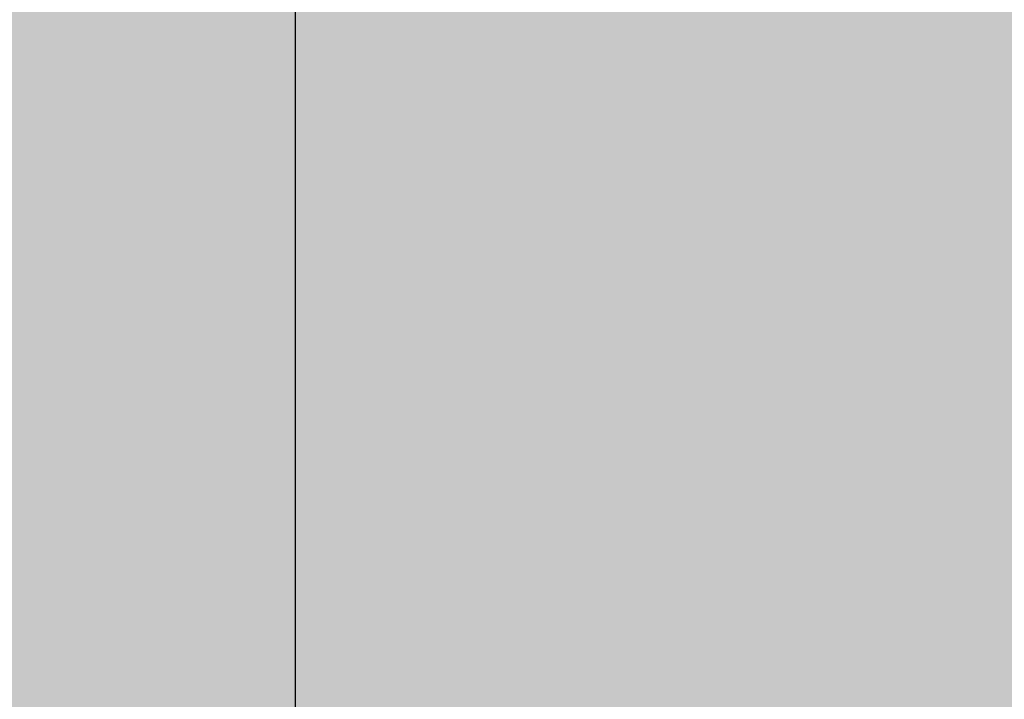
# Model space of a CAD drawing. Units: inches. Extents: x 2083 to 3317, y 1141 to 2115.
# Tile 26 of 256: x 2235.9182 to 2236.0667, y 1477.6562 to 1477.7587. Entities that reach past the tile are written whole.
import ezdxf

# ---------------------------------------------------------------- set-up
doc = ezdxf.new("R2010")
doc.units = ezdxf.units.IN
doc.layers.add('A-ANNO-DIMS', color=2, linetype='Continuous', lineweight=18)
doc.layers.add('A-WALL-PATT', color=251, linetype='Continuous', lineweight=13, true_color=0x636466)
doc.styles.get("Standard").update_dxf_attribs({"font": 'arial.ttf'})
doc.dimstyles.new('ISO-25', dxfattribs={"dimtxt": 12, "dimasz": 12, "dimexe": 1.25, "dimexo": 0.625, "dimtad": 1, "dimlunit": 3, "dimtxsty": 'Standard', "dimcen": 2.5, "dimadec": 0, "dimazin": 0, "dimtfac": 1, "dimtmove": 0, "dimatfit": 3, "dimfxl": 1, "dimarcsym": 0})

# ---------------------------------------------------------------- blocks, each defined once
blk = doc.blocks.new('*D30')
at = {"layer": 'A-ANNO-DIMS', "color": 0, "lineweight": -2, "transparency": 16777216}
for p, q in [((2240.01786, 1445.27381), (2240.01786, 1448.04553)), ((2254.32933, 1445.27381), (2254.32933, 1448.04553)), ((2228.01786, 1446.79553), (2216.01786, 1446.79553)), ((2240.01786, 1446.79553), (2254.32933, 1446.79553)), ((2266.32933, 1446.79553), (2413.76487, 1446.79553))]:
    blk.add_line(p, q, dxfattribs=at)
at = {"layer": 'A-ANNO-DIMS', "color": 0, "transparency": 16777216}
for points in [[(2228.01786, 1448.79553), (2228.01786, 1444.79553), (2240.01786, 1446.79553)], [(2266.32933, 1448.79553), (2266.32933, 1444.79553), (2254.32933, 1446.79553)]]:
    blk.add_solid(points, dxfattribs=at)
at = {"layer": 'Defpoints', "color": 0, "transparency": 16777216}
for p in [(2254.32933, 1446.79553), (2240.01786, 1444.64881), (2254.32933, 1444.64881)]:
    blk.add_point(p, dxfattribs=at)
at = {"layer": 'A-ANNO-DIMS', "color": 0, "transparency": 16777216, "insert": (2346.0471, 1453.62517), "char_height": 12, "attachment_point": 5}
blk.add_mtext('WC 1\'-2 1/2" TYP.', dxfattribs=at)
blk = doc.blocks.new('*D31')
at = {"layer": 'A-ANNO-DIMS', "color": 0, "lineweight": -2, "transparency": 16777216}
for p, q in [((2237.87114, 1456.64881), (2237.87114, 1541.91518)), ((2239.39286, 1444.64881), (2236.62114, 1444.64881)), ((2237.87114, 1431.54754), (2237.87114, 1444.64881)), ((2239.39286, 1431.54754), (2236.62114, 1431.54754)), ((2237.87114, 1419.54754), (2237.87114, 1407.54754))]:
    blk.add_line(p, q, dxfattribs=at)
at = {"layer": 'A-ANNO-DIMS', "color": 0, "transparency": 16777216}
for points in [[(2235.87114, 1456.64881), (2239.87114, 1456.64881), (2237.87114, 1444.64881)], [(2235.87114, 1419.54754), (2239.87114, 1419.54754), (2237.87114, 1431.54754)]]:
    blk.add_solid(points, dxfattribs=at)
at = {"layer": 'Defpoints', "color": 0, "transparency": 16777216}
for p in [(2237.87114, 1444.64881), (2240.01786, 1444.64881), (2240.01786, 1431.54754)]:
    blk.add_point(p, dxfattribs=at)
at = {"layer": 'A-ANNO-DIMS', "color": 0, "transparency": 16777216, "insert": (2231.21749, 1505.28199), "char_height": 12, "attachment_point": 5, "rotation": 90}
blk.add_mtext('1\'-1" TYP.', dxfattribs=at)
blk = doc.blocks.new('*D62')
at = {"layer": 'A-ANNO-DIMS', "color": 0, "lineweight": -2, "transparency": 16777216}
for p, q in [((2235.95978, 1469.38636), (2235.95978, 1522.36136)), ((2379.95978, 1469.38636), (2379.95978, 1522.36136)), ((2247.95978, 1521.11136), (2367.95978, 1521.11136))]:
    blk.add_line(p, q, dxfattribs=at)
at = {"layer": 'A-ANNO-DIMS', "color": 0, "transparency": 16777216}
for points in [[(2247.95978, 1523.11136), (2247.95978, 1519.11136), (2235.95978, 1521.11136)], [(2367.95978, 1523.11136), (2367.95978, 1519.11136), (2379.95978, 1521.11136)]]:
    blk.add_solid(points, dxfattribs=at)
at = {"layer": 'Defpoints', "color": 0, "transparency": 16777216}
for p in [(2379.95978, 1521.11136), (2235.95978, 1468.76136), (2379.95978, 1468.76136)]:
    blk.add_point(p, dxfattribs=at)
at = {"layer": 'A-ANNO-DIMS', "color": 0, "transparency": 16777216, "insert": (2307.95978, 1527.86324), "char_height": 12, "attachment_point": 5}
blk.add_mtext('12\'-0"', dxfattribs=at)

msp = doc.modelspace()

# ---------------------------------------------------------------- hatches: boundary and pattern name
at = {"layer": 'A-WALL-PATT'}
h = msp.add_hatch(color=256, dxfattribs=at)
h.dxf.hatch_style = 1
h.paths.add_polyline_path([(3126.95978, 2020.76136), (2748.95978, 2020.76136), (2604.95978, 2020.76136), (2226.95978, 2020.76136), (2226.95978, 1702.76136), (2466.95978, 1702.76136), (2466.95978, 1582.76136), (2418.95978, 1582.76136), (2418.95978, 1477.76136), (2226.95978, 1477.76136), (2226.95978, 1263.26136), (2544.95978, 1263.26136), (2544.95978, 1411.76136), (2604.95978, 1411.76136), (2685.95978, 1411.76136), (2685.95978, 1420.76136), (2604.95978, 1420.76136), (2604.95978, 1573.76136), (2604.95978, 1702.76136), (2604.95978, 2011.76136), (2748.95978, 2011.76136), (2748.95978, 1702.76136), (2862.95978, 1702.76136), (2862.95978, 1621.76136), (2871.95978, 1621.76136), (2871.95978, 1702.76136), (2883.95978, 1702.76136), (2883.95978, 1706.93946, -0.026459), (2883.95978, 1711.76136), (2757.95978, 1711.76136), (2757.95978, 1807.76136), (2787.95978, 1807.76136), (2787.95978, 1812.26136), (2757.95978, 1812.26136), (2757.95978, 2011.76136), (2877.95978, 2011.76136), (2877.95978, 1812.26136), (2847.95978, 1812.26136), (2847.95978, 1807.76136), (2889.83574, 1807.76136), (2889.83574, 1812.26136), (2882.45978, 1812.26136), (2882.45978, 2011.76136), (3117.95978, 2011.76136), (3117.95978, 1812.26136), (2937.83574, 1812.26136), (2937.83574, 1807.76136), (2995.70978, 1807.76136), (2995.70978, 1796.11767), (3000.20978, 1796.11767), (3000.20978, 1807.76136), (3117.95978, 1807.76136), (3117.95978, 1711.76136), (3000.20978, 1711.76136), (3000.20978, 1760.11767), (2998.5727, 1760.11767, -0.020711), (2995.70978, 1760.11767), (2995.70978, 1711.76136), (2931.95978, 1711.76136), (2931.95978, 1702.76136), (3126.95978, 1702.76136)])
h.paths.add_polyline_path([(2471.45978, 2011.76136), (2471.45978, 1810.01136), (2462.71694, 1810.01136), (2462.71694, 1805.51136), (2505.95978, 1805.51136), (2505.95978, 1810.01136), (2475.95978, 1810.01136), (2475.95978, 2011.76136), (2595.95978, 2011.76136), (2595.95978, 1810.01136), (2565.95978, 1810.01136), (2565.95978, 1805.51136), (2595.95978, 1805.51136), (2595.95978, 1711.76136), (2235.95978, 1711.76136), (2235.95978, 1805.51136), (2353.70978, 1805.51136), (2353.70978, 1796.05416), (2358.20978, 1796.05416), (2358.20978, 1805.51136), (2414.71694, 1805.51136), (2414.71694, 1810.01136), (2235.95978, 1810.01136), (2235.95978, 2011.76136)], flags=16)
h.paths.add_polyline_path([(2270.20473, 1994.61001), (2270.20473, 1970.61001), (2246.20473, 1970.61001), (2246.20473, 1994.61001)], flags=0)
edge = h.paths.add_edge_path(flags=0)
edge.add_ellipse((2332.02739, 1899.79818), major_axis=(-3.04299, 3.04299), ratio=0.1682525, start_angle=-161.33217, end_angle=-156.30711, ccw=False)
edge.add_ellipse((2333.08204, 1898.74353), major_axis=(-1.05465, 1.05465), ratio=0.4535321, start_angle=-123.37102, end_angle=-94.15911)
edge = h.paths.add_edge_path(flags=0)
edge.add_ellipse((2332.02739, 1968.87629), major_axis=(3.04299, 3.04299), ratio=0.1682525, start_angle=18.66783, end_angle=23.69289)
edge.add_spline(control_points=[(2332.9256, 1970.6911), (2332.22677, 1970.3361), (2330.89371, 1969.65891), (2328.41308, 1970.93214), (2327.20393, 1967.74871), (2324.7096, 1969.95559), (2322.53282, 1967.01235), (2320.01285, 1971.29581), (2317.68031, 1968.15784), (2316.04053, 1967.10205), (2315.4269, 1966.8096)], knot_values=[0, 0, 0, 0, 2.267059, 4.324559, 6.685584, 8.878641, 11.121502, 14.300359, 17.755284, 19.732645, 19.732645, 19.732645, 19.732645], degree=3, periodic=0)
edge.add_ellipse((2332.02739, 1968.87629), major_axis=(3.04299, 3.04299), ratio=0.1682525, start_angle=18.66783, end_angle=23.69289, ccw=False)
edge.add_ellipse((2333.08204, 1969.93094), major_axis=(1.05465, 1.05465), ratio=0.4535321, start_angle=56.62898, end_angle=85.84089, ccw=False)
edge = h.paths.add_edge_path(flags=0)
edge.add_spline(control_points=[(2296.42829, 1967.98791), (2293.6278, 1965.33631), (2287.70362, 1959.72709), (2299.74386, 1949.9957), (2294.53259, 1935.66853), (2290.57323, 1920.60351), (2293.39412, 1909.97369), (2296.18541, 1904.96654)], knot_values=[0.099185, 0.099185, 0.099185, 0.099185, 0.345301, 0.619822, 0.982653, 1.386093, 1.810555, 1.810555, 1.810555, 1.810555], degree=3, periodic=0)
edge.add_spline(control_points=[(2296.18541, 1904.96654), (2297.38358, 1902.6193), (2298.00097, 1901.94931), (2298.55297, 1901.46815)], knot_values=[0.006246, 0.006246, 0.006246, 0.006246, 0.055476, 0.055476, 0.055476, 0.055476], degree=3, periodic=0)
edge.add_spline(control_points=[(2298.55297, 1901.46815), (2297.25861, 1900.92322), (2295.22529, 1900.23213), (2293.06023, 1900.61421), (2292.10142, 1900.78841), (2292.08958, 1900.79057)], knot_values=[0.312835, 0.312835, 0.312835, 0.312835, 0.40178, 0.474987, 0.475903, 0.475903, 0.475903, 0.475903], degree=3, periodic=0)
edge.add_arc((2292.79365, 1904.66411), 3.93701, 215.4209, 259.69818, ccw=False)
edge.add_spline(control_points=[(2289.58531, 1902.3823), (2289.47665, 1902.53509), (2289.36848, 1902.68804), (2289.26086, 1902.84117)], knot_values=[0.102872, 0.102872, 0.102872, 0.102872, 0.116896, 0.116896, 0.116896, 0.116896], degree=3, periodic=0)
edge.add_spline(control_points=[(2289.26086, 1902.84117), (2288.6866, 1902.55019), (2287.64005, 1902.0199), (2285.88134, 1901.87395), (2283.85297, 1901.50435), (2281.71999, 1899.71054), (2278.46699, 1899.49294), (2276.15714, 1901.8832), (2272.25895, 1899.80407), (2267.77761, 1901.84318), (2262.24388, 1900.18403), (2257.41493, 1901.78206), (2254.31837, 1900.72612), (2253.17828, 1900.33734)], knot_values=[0, 0, 0, 0, 1.907977, 3.477176, 5.261074, 7.972851, 11.680248, 13.717921, 16.939592, 22.789562, 27.502503, 33.595215, 37.145618, 37.145618, 37.145618, 37.145618], degree=3, periodic=0)
edge.add_line((2253.17828, 1900.33734), (2250.24424, 1902.84117))
edge.add_line((2250.24424, 1902.84117), (2250.24424, 1965.8333))
edge.add_line((2250.24424, 1965.8333), (2253.17828, 1968.33712))
edge.add_spline(control_points=[(2253.17828, 1968.33712), (2254.31837, 1967.94835), (2257.41493, 1966.89241), (2262.24388, 1968.49043), (2267.77761, 1966.83128), (2271.52673, 1968.53722), (2273.87591, 1967.82829), (2274.2067, 1967.72764)], knot_values=[0, 0, 0, 0, 0.09018, 0.244935, 0.364644, 0.513233, 0.537855, 0.537855, 0.537855, 0.537855], degree=3, periodic=0)
edge.add_arc((2274.35289, 1963.79335), 3.93701, 72.05113, 92.12795, ccw=False)
edge.add_arc((2281.29693, 1985.23), 18.5963, 252.051134, 288.565722)
edge.add_arc((2292.31672, 1956.02888), 12.64608, 71.026788, 113.778218, ccw=False)
edge = h.paths.add_edge_path(flags=0)
edge.add_spline(control_points=[(2274.89941, 1951.85619), (2275.06616, 1951.61659), (2275.23269, 1951.37659), (2275.39799, 1951.13585)], knot_values=[1.409916, 1.409916, 1.409916, 1.409916, 1.43159, 1.43159, 1.43159, 1.43159], degree=3, periodic=0)
edge.add_spline(control_points=[(2275.39799, 1951.13585), (2275.79211, 1950.56189), (2276.17923, 1949.98377), (2276.54555, 1949.3971)], knot_values=[1.358238, 1.358238, 1.358238, 1.358238, 1.409916, 1.409916, 1.409916, 1.409916], degree=3, periodic=0)
edge.add_line((2276.54555, 1949.3971), (2277.43729, 1947.86218))
edge.add_spline(control_points=[(2277.43729, 1947.86218), (2276.30383, 1945.67311), (2274.6397, 1942.42688), (2274.63161, 1938.0939), (2272.79912, 1930.85155), (2274.35643, 1943.89705), (2275.94768, 1947.92336), (2276.54555, 1949.3971)], knot_values=[0.005632, 0.005632, 0.005632, 0.005632, 0.186014, 0.266002, 0.357087, 0.59639, 0.739732, 0.739732, 0.739732, 0.739732], degree=3, periodic=0)
edge.add_spline(control_points=[(2276.54555, 1949.3971), (2276.17923, 1949.98377), (2275.79211, 1950.56189), (2275.39799, 1951.13585)], knot_values=[1.358238, 1.358238, 1.358238, 1.358238, 1.409916, 1.409916, 1.409916, 1.409916], degree=3, periodic=0)
edge.add_spline(control_points=[(2275.39799, 1951.13585), (2274.9425, 1950.08045), (2274.20776, 1948.02527), (2273.9346, 1944.85148), (2272.46853, 1937.62749), (2273.46622, 1945.69647), (2274.70062, 1951.05947), (2274.89941, 1951.85619)], knot_values=[0.104364, 0.104364, 0.104364, 0.104364, 0.189636, 0.269624, 0.36071, 0.600013, 0.644622, 0.644622, 0.644622, 0.644622], degree=3, periodic=0)
h.paths.add_polyline_path([(2269.16751, 1963.12757, -0.357527), (2268.17063, 1960.97637, -0.092561), (2268.17063, 1939.43632, -0.357527), (2269.16751, 1937.28512, -0.357527), (2267.01631, 1938.282, -0.164785), (2254.68558, 1938.282, -0.357527), (2252.53438, 1937.28512, -0.357527), (2253.53126, 1939.43632, -0.092561), (2253.53126, 1960.97637, -0.357527), (2252.53438, 1963.12757, -0.357527), (2254.68558, 1962.13069, -0.164785), (2267.01631, 1962.13069, -0.357527)], flags=0)
h.paths.add_polyline_path([(2248.87407, 1967.8018), (2248.87407, 1957.02771), (2249.45778, 1957.02771), (2249.45778, 1911.64676), (2248.87407, 1911.64676), (2248.87407, 1900.87267), (2246.51186, 1900.87267, 0.197327), (2244.14966, 1902.45687), (2244.14966, 1966.21759, 0.197327), (2246.51186, 1967.8018)], flags=0)
h.paths.add_polyline_path([(2269.16751, 1931.38934, -0.357527), (2268.17063, 1929.23814, -0.092561), (2268.17063, 1907.6981, -0.357527), (2269.16751, 1905.54689, -0.357527), (2267.01631, 1906.54377, -0.164785), (2254.68558, 1906.54377, -0.357527), (2252.53438, 1905.54689, -0.357527), (2253.53126, 1907.6981, -0.092561), (2253.53126, 1929.23814, -0.357527), (2252.53438, 1931.38934, -0.357527), (2254.68558, 1930.39246, -0.164785), (2267.01631, 1930.39246, -0.357527)], flags=0)
edge = h.paths.add_edge_path(flags=0)
edge.add_spline(control_points=[(2276.19686, 1906.7237), (2276.16814, 1909.02893), (2276.11405, 1913.37185), (2270.59842, 1924.92498), (2273.90517, 1919.01278), (2275.92171, 1916.26206), (2275.47457, 1912.40215), (2277.25787, 1910.38062), (2276.69604, 1908.22504), (2276.64622, 1906.81302), (2276.61782, 1906.00841)], knot_values=[0, 0, 0, 0, 8.61026, 16.221274, 18.843057, 23.804898, 27.440828, 29.356102, 31.203478, 33.650687, 33.650687, 33.650687, 33.650687], degree=3, periodic=0)
edge.add_spline(control_points=[(2276.61782, 1906.00841), (2276.62331, 1905.62414), (2276.49774, 1904.62866), (2275.44178, 1903.85473), (2274.93731, 1903.08045), (2274.85908, 1902.84117)], knot_values=[0.156488, 0.156488, 0.156488, 0.156488, 0.184398, 0.231376, 0.250598, 0.250598, 0.250598, 0.250598], degree=3, periodic=0)
edge.add_line((2274.85908, 1902.84117), (2276.50598, 1902.84117))
edge.add_spline(control_points=[(2276.50598, 1902.84117), (2276.78831, 1903.08494), (2277.66507, 1904.1252), (2278.24954, 1904.34074), (2277.65387, 1908.52739), (2278.15567, 1906.22781), (2278.10046, 1905.28595), (2278.84667, 1904.06901), (2277.85679, 1903.41495), (2277.87419, 1902.99105), (2277.90356, 1902.84117)], knot_values=[0.059574, 0.059574, 0.059574, 0.059574, 0.080753, 0.103741, 0.16972, 0.176036, 0.207137, 0.240474, 0.262341, 0.27366, 0.27366, 0.27366, 0.27366], degree=3, periodic=0)
edge.add_line((2277.90356, 1902.84117), (2280.02983, 1902.84117))
edge.add_spline(control_points=[(2280.02983, 1902.84117), (2279.88822, 1903.0884), (2279.49926, 1903.98155), (2280.15228, 1905.93935), (2278.10362, 1909.65776), (2279.76239, 1907.18529), (2280.3279, 1904.87486), (2280.48511, 1903.48959), (2281.46327, 1903.24943), (2281.75834, 1902.9365), (2281.83404, 1902.84117)], knot_values=[0.013856, 0.013856, 0.013856, 0.013856, 0.034874, 0.088867, 0.107879, 0.126738, 0.158714, 0.193757, 0.217487, 0.226722, 0.226722, 0.226722, 0.226722], degree=3, periodic=0)
edge.add_spline(control_points=[(2281.83404, 1902.84117), (2281.78753, 1902.8267), (2281.64702, 1902.78299), (2281.39553, 1902.85949), (2281.08808, 1902.98524), (2280.72068, 1903.0609), (2280.33345, 1903.02573), (2280.12477, 1902.89888), (2280.02983, 1902.84117)], knot_values=[0, 0, 0, 0, 0.14413, 0.435517, 0.749276, 1.153046, 1.548371, 1.878348, 1.878348, 1.878348, 1.878348], degree=3, periodic=0)
edge.add_line((2280.02983, 1902.84117), (2277.90356, 1902.84117))
edge.add_spline(control_points=[(2277.90356, 1902.84117), (2277.89286, 1902.79586), (2277.8654, 1902.67964), (2277.60748, 1902.68748), (2277.27405, 1902.8007), (2276.83792, 1902.61977), (2276.58381, 1902.78926), (2276.50598, 1902.84117)], knot_values=[0, 0, 0, 0, 0.127189, 0.326199, 0.628009, 1.24357, 1.515331, 1.515331, 1.515331, 1.515331], degree=3, periodic=0)
edge.add_line((2276.50598, 1902.84117), (2274.85908, 1902.84117))
edge.add_spline(control_points=[(2274.85908, 1902.84117), (2274.81444, 1902.89859), (2274.72513, 1903.01345), (2274.49348, 1903.11897), (2274.24429, 1902.96054), (2273.93712, 1903.18494), (2273.61404, 1902.98314), (2273.40832, 1902.88304), (2273.32225, 1902.84117)], knot_values=[0, 0, 0, 0, 0.21843, 0.436957, 0.687977, 0.990379, 1.398396, 1.69185, 1.69185, 1.69185, 1.69185], degree=3, periodic=0)
edge.add_spline(control_points=[(2273.32225, 1902.84117), (2273.61674, 1903.44569), (2274.274, 1904.53825), (2276.02724, 1904.5737), (2276.20696, 1906.58364), (2276.19686, 1906.7237)], knot_values=[0.012227, 0.012227, 0.012227, 0.012227, 0.059472, 0.106218, 0.134458, 0.134458, 0.134458, 0.134458], degree=3, periodic=0)
h.paths.add_polyline_path([(2270.77605, 1897.78983), (2270.77605, 1873.78983), (2246.77605, 1873.78983), (2246.77605, 1897.78983)], flags=0)
h.paths.add_polyline_path([(2353.70978, 1760.00506), (2353.70978, 1760.05416), (2358.20978, 1760.05416, -0.033729)], flags=0)
h.paths.add_polyline_path([(2321.81912, 1737.52919), (2341.99533, 1737.52919, -0.414214), (2343.20327, 1736.32124), (2343.20327, 1721.0206, -0.414214), (2341.99533, 1719.81265), (2321.81912, 1719.81265, -0.414214), (2320.61117, 1721.0206), (2320.61117, 1736.32124, -0.414214)], flags=0)
h.paths.add_polyline_path([(2324.23501, 1736.32124), (2339.57944, 1736.32124, -0.414214), (2341.99533, 1733.90535), (2341.99533, 1725.44973, -0.414214), (2339.57944, 1723.03384), (2333.68059, 1723.03384), (2333.84532, 1722.04547, -0.870646), (2335.4254, 1721.82589, -0.767327), (2333.92269, 1721.42324), (2331.29102, 1721.42324, -0.767327), (2329.78832, 1721.82589, -0.870646), (2331.3684, 1722.04547), (2331.53313, 1723.03384), (2324.23501, 1723.03384, -0.414214), (2321.81912, 1725.44973), (2321.81912, 1733.90535, -0.414214)], flags=0)
h.paths.add_polyline_path([(2570.48379, 1928.61544), (2589.68379, 1928.61544), (2590.16883, 1928.61544), (2590.16883, 1904.9934), (2570.48379, 1904.9934)], flags=0)
h.paths.add_polyline_path([(2574.44732, 1927.26382, -1), (2572.82884, 1927.26382, -1)], flags=0)
h.paths.add_polyline_path([(2573.08987, 1926.94088), (2573.92503, 1927.77604), (2574.14774, 1927.55333), (2573.31258, 1926.71817)], flags=0)
h.paths.add_polyline_path([(2578.77906, 1919.72962, -1), (2571.59166, 1919.72962, -1)], flags=0)
h.paths.add_polyline_path([(2578.38536, 1919.72962, -1), (2571.98536, 1919.72962, -1)], flags=0)
h.paths.add_polyline_path([(2331.59576, 1729.47622, -1), (2333.61795, 1729.47622, -1)], flags=0)
h.paths.add_polyline_path([(2578.03423, 1927.26382, -1), (2576.41574, 1927.26382, -1)], flags=0)
h.paths.add_polyline_path([(2576.68885, 1927.53109), (2576.91156, 1927.7538), (2577.74673, 1926.91863), (2577.52402, 1926.69592)], flags=0)
h.paths.add_polyline_path([(2578.13906, 1909.85954, -1), (2572.23166, 1909.85954, -1)], flags=0)
h.paths.add_polyline_path([(2577.74536, 1909.85954, -1), (2572.62536, 1909.85954, -1)], flags=0)
h.paths.add_polyline_path([(2583.79772, 1927.26382, -1), (2582.17923, 1927.26382, -1)], flags=0)
h.paths.add_polyline_path([(2582.71865, 1927.7538), (2583.55381, 1926.91863), (2583.3311, 1926.69592), (2582.49594, 1927.53109)], flags=0)
h.paths.add_polyline_path([(2582.49594, 1927.53109), (2582.71865, 1927.7538), (2583.55381, 1926.91863), (2583.3311, 1926.69592)], flags=0)
h.paths.add_polyline_path([(2587.73906, 1920.52962, -1), (2581.83166, 1920.52962, -1)], flags=0)
h.paths.add_polyline_path([(2587.34536, 1920.52962, -1), (2582.22536, 1920.52962, -1)], flags=0)
h.paths.add_polyline_path([(2587.38462, 1927.26382, -1), (2585.76613, 1927.26382, -1)], flags=0)
h.paths.add_polyline_path([(2586.08199, 1926.98025), (2586.91716, 1927.81541), (2587.13987, 1927.5927), (2586.3047, 1926.75754)], flags=0)
h.paths.add_polyline_path([(2588.37906, 1910.65954, -1), (2581.19166, 1910.65954, -1)], flags=0)
h.paths.add_polyline_path([(2587.98536, 1910.65954, -1), (2581.58536, 1910.65954, -1)], flags=0)
h.paths.add_polyline_path([(2417.16773, 1729.4779), (2437.34394, 1729.4779, -0.414214), (2438.55188, 1728.26995), (2438.55188, 1712.96931, -0.414214), (2437.34394, 1711.76136), (2417.16773, 1711.76136, -0.414214), (2415.95978, 1712.96931), (2415.95978, 1728.26995, -0.414214)], flags=0)
h.paths.add_polyline_path([(2419.58362, 1728.26995), (2434.92805, 1728.26995, -0.414214), (2437.34394, 1725.85406), (2437.34394, 1717.39844, -0.414214), (2434.92805, 1714.98255), (2429.0292, 1714.98255), (2429.19393, 1713.99418, -0.870646), (2430.77401, 1713.7746, -0.767327), (2429.2713, 1713.37195), (2426.63963, 1713.37195, -0.767327), (2425.13693, 1713.7746, -0.870646), (2426.71701, 1713.99418), (2426.88174, 1714.98255), (2419.58362, 1714.98255, -0.414214), (2417.16773, 1717.39844), (2417.16773, 1725.85406, -0.414214)], flags=0)
h.paths.add_polyline_path([(2419.58362, 1728.26995), (2434.92805, 1728.26995, -0.414214), (2437.34394, 1725.85406), (2437.34394, 1717.39844, -0.414214), (2434.92805, 1714.98255), (2429.0292, 1714.98255), (2428.35812, 1719.00903), (2427.55282, 1719.00903), (2426.88174, 1714.98255), (2419.58362, 1714.98255, -0.414214), (2417.16773, 1717.39844), (2417.16773, 1725.85406, -0.414214)], flags=0)
h.paths.add_polyline_path([(2426.94437, 1721.42492, -1), (2428.96656, 1721.42492, -1)], flags=0)
h.paths.add_polyline_path([(2475.95978, 1702.76136), (2595.95978, 1702.76136), (2595.95978, 1582.76136), (2475.95978, 1582.76136)], flags=16)
h.paths.add_polyline_path([(2427.95978, 1573.76136), (2595.95978, 1573.76136), (2595.95978, 1468.76136), (2595.95978, 1420.76136), (2384.45978, 1420.76136), (2384.45978, 1468.76136), (2427.95978, 1468.76136)], flags=16)
h.paths.add_polyline_path([(2379.95978, 1468.76136), (2379.95978, 1420.76136), (2235.95978, 1420.76136), (2235.95978, 1468.76136)], flags=16)
h.paths.add_polyline_path([(2317.816, 1466.69577), (2337.9922, 1466.69577, -0.414214), (2339.20015, 1465.48782), (2339.20015, 1450.18718, -0.414214), (2337.9922, 1448.97923), (2317.816, 1448.97923, -0.414214), (2316.60805, 1450.18718), (2316.60805, 1465.48782, -0.414214)], flags=0)
h.paths.add_polyline_path([(2320.23189, 1465.48782), (2335.57631, 1465.48782, -0.414214), (2337.9922, 1463.07193), (2337.9922, 1454.61631, -0.414214), (2335.57631, 1452.20042), (2329.67747, 1452.20042), (2329.84219, 1451.21205, -0.870646), (2331.42228, 1450.99247, -0.767327), (2329.91957, 1450.58983), (2327.2879, 1450.58983, -0.767327), (2325.7852, 1450.99247, -0.870646), (2327.36528, 1451.21205), (2327.53001, 1452.20042), (2320.23189, 1452.20042, -0.414214), (2317.816, 1454.61631), (2317.816, 1463.07193, -0.414214)], flags=0)
h.paths.add_polyline_path([(2320.23189, 1465.48782), (2335.57631, 1465.48782, -0.414214), (2337.9922, 1463.07193), (2337.9922, 1454.61631, -0.414214), (2335.57631, 1452.20042), (2329.67747, 1452.20042), (2329.00638, 1456.22691), (2328.20109, 1456.22691), (2327.53001, 1452.20042), (2320.23189, 1452.20042, -0.414214), (2317.816, 1454.61631), (2317.816, 1463.07193, -0.414214)], flags=0)
h.paths.add_polyline_path([(2327.59264, 1458.6428, -1), (2329.61483, 1458.6428, -1)], flags=0)
h.paths.add_polyline_path([(2244.41174, 1433.34045), (2241.92094, 1433.34045, -0.414214), (2240.01786, 1435.24354), (2240.01786, 1440.95281, -0.414211), (2241.92093, 1442.8559), (2244.41174, 1442.8559, -1.976472)], flags=0)
h.paths.add_polyline_path([(2245.35689, 1434.39754, -0.414214), (2245.35689, 1441.79881, -2.144098)], flags=0)
h.paths.add_polyline_path([(2535.95978, 1416.26136), (2535.95978, 1272.26136), (2235.95978, 1272.26136), (2235.95978, 1416.26136)], flags=16)
h.paths.add_polyline_path([(2260.11956, 1384.29284), (2260.11956, 1362.03865), (2237.86537, 1362.03865), (2237.86537, 1384.29284)], flags=0)
edge = h.paths.add_edge_path(flags=0)
edge.add_line((2318.25185, 1362.0933), (2318.1458, 1362.00097))
edge.add_ellipse((2317.44512, 1360.43104), major_axis=(2.82164, 2.82164), ratio=0.1682525, start_angle=18.66783, end_angle=20.94813, ccw=False)
edge.add_ellipse((2318.42305, 1361.40897), major_axis=(0.97793, 0.97793), ratio=0.4535321, start_angle=56.62898, end_angle=70.2262, ccw=False)
edge = h.paths.add_edge_path(flags=0)
edge.add_line((2319.10737, 1295.57108), (2319.01504, 1295.67713))
edge.add_ellipse((2317.44512, 1296.37781), major_axis=(-2.82164, 2.82164), ratio=0.1682525, start_angle=-161.33217, end_angle=-159.05187, ccw=False)
edge.add_ellipse((2318.42305, 1295.39988), major_axis=(-0.97793, 0.97793), ratio=0.4535321, start_angle=-123.37102, end_angle=-109.7738)
edge = h.paths.add_edge_path(flags=0)
edge.add_spline(control_points=[(2284.21035, 1301.17022), (2284.58069, 1300.44472), (2284.89119, 1299.89202), (2285.15955, 1299.46102)], knot_values=[0.039066, 0.039066, 0.039066, 0.039066, 0.055476, 0.055476, 0.055476, 0.055476], degree=3, periodic=0)
edge.add_line((2285.15955, 1299.46102), (2284.21035, 1301.17022))
edge = h.paths.add_edge_path(flags=0)
edge.add_line((2280.41246, 1297.29801), (2283.36999, 1297.03612))
edge.add_line((2283.36999, 1297.03612), (2286.40569, 1297.92631))
edge.add_spline(control_points=[(2286.40569, 1297.92631), (2285.30549, 1297.46312), (2284.34478, 1297.12915), (2283.36999, 1297.03612)], knot_values=[0.394369, 0.394369, 0.394369, 0.394369, 0.475903, 0.475903, 0.475903, 0.475903], degree=3, periodic=0)
edge.add_spline(control_points=[(2283.36999, 1297.03612), (2283.28139, 1297.02767), (2282.31629, 1296.95734), (2281.3125, 1297.13448), (2280.42344, 1297.29602), (2280.41246, 1297.29801)], knot_values=[0.312835, 0.312835, 0.312835, 0.312835, 0.320246, 0.393453, 0.394369, 0.394369, 0.394369, 0.394369], degree=3, periodic=0)
edge = h.paths.add_edge_path(flags=0)
edge.add_line((2284.43556, 1359.60729), (2280.44629, 1355.32805))
edge.add_line((2280.44629, 1355.32805), (2279.57999, 1351.01775))
edge.add_line((2279.57999, 1351.01775), (2282.41297, 1346.58043))
edge.add_spline(control_points=[(2282.41297, 1346.58043), (2283.15333, 1345.58924), (2284.2529, 1344.0289), (2284.80104, 1342.38717), (2284.93516, 1341.80554)], knot_values=[1.240098, 1.240098, 1.240098, 1.240098, 1.332892, 1.382712, 1.382712, 1.382712, 1.382712], degree=3, periodic=0)
edge.add_spline(control_points=[(2284.93516, 1341.80554), (2285.31911, 1340.1406), (2285.23303, 1338.4092), (2284.90994, 1336.65412)], knot_values=[1.097484, 1.097484, 1.097484, 1.097484, 1.240098, 1.240098, 1.240098, 1.240098], degree=3, periodic=0)
edge.add_spline(control_points=[(2284.90994, 1336.65412), (2284.58685, 1334.89904), (2284.02675, 1333.12027), (2283.46264, 1331.36058)], knot_values=[0.95487, 0.95487, 0.95487, 0.95487, 1.097484, 1.097484, 1.097484, 1.097484], degree=3, periodic=0)
edge.add_line((2283.46264, 1331.36058), (2281.89038, 1326.15336))
edge.add_line((2281.89038, 1326.15336), (2280.75626, 1321.05609))
edge.add_line((2280.75626, 1321.05609), (2280.2992, 1316.00198))
edge.add_line((2280.2992, 1316.00198), (2280.71593, 1310.95007))
edge.add_line((2280.71593, 1310.95007), (2282.02809, 1305.97214))
edge.add_line((2282.02809, 1305.97214), (2284.21035, 1301.17022))
edge.add_spline(control_points=[(2284.21035, 1301.17022), (2283.34073, 1302.73019), (2282.6119, 1304.33649), (2282.02809, 1305.97214)], knot_values=[0.099185, 0.099185, 0.099185, 0.099185, 0.241799, 0.241799, 0.241799, 0.241799], degree=3, periodic=0)
edge.add_spline(control_points=[(2282.02809, 1305.97214), (2281.44428, 1307.60778), (2281.00549, 1309.27276), (2280.71593, 1310.95007)], knot_values=[0.241799, 0.241799, 0.241799, 0.241799, 0.384413, 0.384413, 0.384413, 0.384413], degree=3, periodic=0)
edge.add_spline(control_points=[(2280.71593, 1310.95007), (2280.43324, 1312.58761), (2280.28939, 1314.27696), (2280.29889, 1315.96203), (2280.2992, 1316.00198)], knot_values=[0.384413, 0.384413, 0.384413, 0.384413, 0.523647, 0.527028, 0.527028, 0.527028, 0.527028], degree=3, periodic=0)
edge.add_spline(control_points=[(2280.2992, 1316.00198), (2280.31233, 1317.68696), (2280.47787, 1319.36793), (2280.75626, 1321.05609)], knot_values=[0.527028, 0.527028, 0.527028, 0.527028, 0.669642, 0.669642, 0.669642, 0.669642], degree=3, periodic=0)
edge.add_spline(control_points=[(2280.75626, 1321.05609), (2281.03465, 1322.74425), (2281.42588, 1324.43961), (2281.89038, 1326.15336)], knot_values=[0.669642, 0.669642, 0.669642, 0.669642, 0.812256, 0.812256, 0.812256, 0.812256], degree=3, periodic=0)
edge.add_spline(control_points=[(2281.89038, 1326.15336), (2282.26438, 1327.53325), (2282.78787, 1329.26181), (2283.35275, 1331.01778), (2283.46264, 1331.36058)], knot_values=[0.812256, 0.812256, 0.812256, 0.812256, 0.927087, 0.95487, 0.95487, 0.95487, 0.95487], degree=3, periodic=0)
edge.add_line((2283.46264, 1331.36058), (2284.90994, 1336.65412))
edge.add_line((2284.90994, 1336.65412), (2284.93516, 1341.80554))
edge.add_line((2284.93516, 1341.80554), (2282.41297, 1346.58043))
edge.add_spline(control_points=[(2282.41297, 1346.58043), (2281.27513, 1348.10379), (2280.07845, 1349.57032), (2279.57999, 1351.01775)], knot_values=[1.382712, 1.382712, 1.382712, 1.382712, 1.525326, 1.525326, 1.525326, 1.525326], degree=3, periodic=0)
edge.add_spline(control_points=[(2279.57999, 1351.01775), (2279.44328, 1351.41472), (2279.13631, 1352.85692), (2279.73519, 1354.29039), (2280.44629, 1355.32805)], knot_values=[1.525326, 1.525326, 1.525326, 1.525326, 1.564439, 1.667941, 1.667941, 1.667941, 1.667941], degree=3, periodic=0)
edge.add_spline(control_points=[(2280.44629, 1355.32805), (2281.42611, 1356.75784), (2282.93084, 1358.18256), (2284.43556, 1359.60729)], knot_values=[1.667941, 1.667941, 1.667941, 1.667941, 1.810555, 1.810555, 1.810555, 1.810555], degree=3, periodic=0)
edge.add_arc((2280.62307, 1348.51818), 11.72618, 71.026788, 113.778218)
edge.add_arc((2270.40489, 1375.59516), 17.24357, 252.051134, 288.565722, ccw=False)
edge.add_arc((2263.96597, 1355.71785), 3.65062, 72.05113, 92.12795)
edge.add_arc((2263.96597, 1355.71785), 3.65062, 92.12795, 177.98513)
edge.add_spline(control_points=[(2260.3176, 1355.8462), (2260.26042, 1354.22067), (2260.55128, 1350.18655), (2262.99934, 1346.76625), (2264.47274, 1344.64902)], knot_values=[1.43159, 1.43159, 1.43159, 1.43159, 1.564144, 1.770695, 1.770695, 1.770695, 1.770695], degree=3, periodic=0)
edge.add_line((2264.47274, 1344.64902), (2264.93559, 1343.98253))
edge.add_spline(control_points=[(2263.80104, 1340.24811), (2263.84324, 1340.51409), (2264.06724, 1341.75647), (2264.51269, 1343.00245), (2264.93505, 1343.98108)], knot_values=[0.53657, 0.53657, 0.53657, 0.53657, 0.559349, 0.644622, 0.644622, 0.644622, 0.644622], degree=3, periodic=0)
edge.add_spline(control_points=[(2264.93505, 1343.98108), (2265.11777, 1343.71497), (2265.29888, 1343.44791), (2265.47676, 1343.17936)], knot_values=[1.384077, 1.384077, 1.384077, 1.384077, 1.409916, 1.409916, 1.409916, 1.409916], degree=3, periodic=0)
edge.add_spline(control_points=[(2265.47676, 1343.17936), (2265.65464, 1342.91082), (2265.8293, 1342.64081), (2265.99913, 1342.36881)], knot_values=[1.358238, 1.358238, 1.358238, 1.358238, 1.384077, 1.384077, 1.384077, 1.384077], degree=3, periodic=0)
edge.add_line((2265.99913, 1342.36881), (2266.82601, 1340.94555))
edge.add_spline(control_points=[(2266.82601, 1340.94555), (2268.8944, 1337.08969), (2271.39817, 1325.843), (2270.51616, 1310.56856), (2275.91938, 1301.86061), (2277.78951, 1299.19945)], knot_values=[0.116896, 0.116896, 0.116896, 0.116896, 0.472987, 1.050969, 1.313793, 1.313793, 1.313793, 1.313793], degree=3, periodic=0)
edge.add_spline(control_points=[(2277.78951, 1299.19945), (2277.83941, 1299.12845), (2277.88943, 1299.0575), (2277.93957, 1298.98658)], knot_values=[0.109884, 0.109884, 0.109884, 0.109884, 0.116896, 0.116896, 0.116896, 0.116896], degree=3, periodic=0)
edge.add_line((2277.93957, 1298.98658), (2277.78885, 1299.19911))
edge.add_spline(control_points=[(2277.78885, 1299.19911), (2277.25658, 1298.92941), (2276.28635, 1298.4379), (2275.03935, 1298.33442), (2274.38333, 1298.2389), (2274.21525, 1298.20934)], knot_values=[33.12187, 33.12187, 33.12187, 33.12187, 35.029056, 36.598255, 37.144827, 37.144827, 37.144827, 37.144827], degree=3, periodic=0)
edge.add_line((2274.21525, 1298.20934), (2273.07315, 1297.89296))
edge.add_spline(control_points=[(2273.07315, 1297.89296), (2272.32294, 1297.57978), (2271.03915, 1296.51051), (2269.24839, 1296.22606), (2268.4231, 1296.37465)], knot_values=[26.532584, 26.532584, 26.532584, 26.532584, 29.198919, 31.839101, 31.839101, 31.839101, 31.839101], degree=3, periodic=0)
edge.add_line((2268.4231, 1296.37465), (2263.8785, 1297.45753))
edge.add_spline(control_points=[(2263.8785, 1297.45753), (2263.55608, 1297.35943), (2261.86031, 1296.83869), (2260.23878, 1297.28241), (2258.93345, 1297.51646)], knot_values=[15.919551, 15.919551, 15.919551, 15.919551, 16.939592, 21.226067, 21.226067, 21.226067, 21.226067], degree=3, periodic=0)
edge.add_line((2258.93345, 1297.51646), (2254.05523, 1297.32901))
edge.add_spline(control_points=[(2254.05523, 1297.32901), (2253.75553, 1297.29582), (2252.11368, 1297.16517), (2250.46187, 1297.54422), (2249.12969, 1297.66788)], knot_values=[5.306517, 5.306517, 5.306517, 5.306517, 6.276435, 10.613034, 10.613034, 10.613034, 10.613034], degree=3, periodic=0)
edge.add_line((2249.12969, 1297.66788), (2244.33165, 1296.87776))
edge.add_line((2244.33165, 1296.87776), (2241.61103, 1299.19945))
edge.add_line((2241.61103, 1299.19945), (2241.61103, 1357.6094))
edge.add_line((2241.61103, 1357.6094), (2244.33165, 1359.9311))
edge.add_line((2244.33165, 1359.9311), (2252.72882, 1359.54269))
edge.add_spline(control_points=[(2252.72882, 1359.54269), (2252.87094, 1359.54644), (2253.30574, 1359.54817), (2253.73984, 1359.51427), (2254.03174, 1359.48243)], knot_values=[0.233291, 0.233291, 0.233291, 0.233291, 0.244935, 0.268927, 0.268927, 0.268927, 0.268927], degree=3, periodic=0)
edge.add_line((2254.03174, 1359.48243), (2259.58719, 1359.41639))
edge.add_spline(control_points=[(2259.58719, 1359.41639), (2260.67707, 1359.6285), (2262.0732, 1359.897), (2263.52369, 1359.45928), (2263.83042, 1359.36595)], knot_values=[0.422516, 0.422516, 0.422516, 0.422516, 0.513233, 0.537855, 0.537855, 0.537855, 0.537855], degree=3, periodic=0)
edge.add_arc((2263.96597, 1355.71785), 3.65062, 72.05113, 92.12795, ccw=False)
edge.add_arc((2270.40489, 1375.59516), 17.24357, 252.051134, 288.565722)
edge.add_arc((2280.62307, 1348.51818), 11.72618, 71.026788, 113.778218, ccw=False)
h.paths.add_polyline_path([(2240.34053, 1359.43471), (2240.34053, 1349.44435), (2240.88178, 1349.44435), (2240.88178, 1307.3645), (2240.34053, 1307.3645), (2240.34053, 1297.37414), (2238.15016, 1297.37414, 0.197327), (2235.95978, 1298.84311), (2235.95978, 1357.96575, 0.197327), (2238.15016, 1359.43471)], flags=0)
h.paths.add_polyline_path([(2259.15779, 1355.1005, -0.357527), (2258.23342, 1353.10578, -0.092561), (2258.23342, 1333.1326, -0.357527), (2259.15779, 1331.13788, -0.357527), (2257.16307, 1332.06225, -0.164785), (2245.7293, 1332.06225, -0.357527), (2243.73458, 1331.13788, -0.357527), (2244.65895, 1333.1326, -0.092561), (2244.65895, 1353.10578, -0.357527), (2243.73458, 1355.1005, -0.357527), (2245.7293, 1354.17613, -0.164785), (2257.16307, 1354.17613, -0.357527)], flags=0)
edge = h.paths.add_edge_path(flags=0)
edge.add_line((2265.99913, 1342.36881), (2266.82601, 1340.94555))
edge.add_line((2266.82601, 1340.94555), (2265.30756, 1337.81407))
edge.add_line((2265.30756, 1337.81407), (2264.35823, 1334.65294))
edge.add_line((2264.35823, 1334.65294), (2264.26201, 1333.7997))
edge.add_spline(control_points=[(2264.26201, 1333.7997), (2264.20836, 1333.18705), (2264.16206, 1332.36553), (2264.00714, 1331.41393), (2263.96905, 1331.20183)], knot_values=[0.464444, 0.464444, 0.464444, 0.464444, 0.516691, 0.531608, 0.531608, 0.531608, 0.531608], degree=3, periodic=0)
edge.add_spline(control_points=[(2263.96905, 1331.20183), (2263.77453, 1330.11887), (2263.42437, 1328.79084), (2263.25742, 1328.53065), (2263.23403, 1328.51461)], knot_values=[0.372682, 0.372682, 0.372682, 0.372682, 0.44885, 0.464444, 0.464444, 0.464444, 0.464444], degree=3, periodic=0)
edge.add_spline(control_points=[(2263.23403, 1328.51461), (2263.09638, 1328.42023), (2263.13117, 1329.30148), (2263.27495, 1330.61575)], knot_values=[0.280919, 0.280919, 0.280919, 0.280919, 0.372682, 0.372682, 0.372682, 0.372682], degree=3, periodic=0)
edge.add_spline(control_points=[(2263.27495, 1330.61575), (2263.41874, 1331.93002), (2263.67152, 1333.67732), (2263.96985, 1335.31503)], knot_values=[0.189157, 0.189157, 0.189157, 0.189157, 0.280919, 0.280919, 0.280919, 0.280919], degree=3, periodic=0)
edge.add_spline(control_points=[(2263.96985, 1335.31503), (2264.1005, 1336.03219), (2264.41878, 1337.62191), (2264.75485, 1338.86443), (2264.94742, 1339.49112)], knot_values=[0.097394, 0.097394, 0.097394, 0.097394, 0.137578, 0.189157, 0.189157, 0.189157, 0.189157], degree=3, periodic=0)
edge.add_spline(control_points=[(2264.94742, 1339.49112), (2265.29002, 1340.60605), (2265.64424, 1341.494), (2265.99913, 1342.36881)], knot_values=[0.005632, 0.005632, 0.005632, 0.005632, 0.097394, 0.097394, 0.097394, 0.097394], degree=3, periodic=0)
h.paths.add_polyline_path([(2259.15779, 1325.67097, -0.357527), (2258.23342, 1323.67625, -0.092561), (2258.23342, 1303.70307, -0.357527), (2259.15779, 1301.70835, -0.357527), (2257.16307, 1302.63272, -0.164785), (2245.7293, 1302.63272, -0.357527), (2243.73458, 1301.70835, -0.357527), (2244.65895, 1303.70307, -0.092561), (2244.65895, 1323.67625, -0.357527), (2243.73458, 1325.67097, -0.357527), (2245.7293, 1324.74661, -0.164785), (2257.16307, 1324.74661, -0.357527)], flags=0)
edge = h.paths.add_edge_path(flags=0)
edge.add_spline(control_points=[(2261.70894, 1317.31142), (2261.67948, 1317.41758), (2261.76186, 1317.38853), (2262.49074, 1316.08987), (2262.96218, 1315.3009)], knot_values=[14.955861, 14.955861, 14.955861, 14.955861, 16.221274, 18.694826, 18.694826, 18.694826, 18.694826], degree=3, periodic=0)
edge.add_spline(control_points=[(2262.96218, 1315.3009), (2262.99044, 1315.25362), (2263.7021, 1314.06738), (2264.34898, 1313.12715), (2264.73005, 1312.16415)], knot_values=[18.694826, 18.694826, 18.694826, 18.694826, 18.843057, 22.433791, 22.433791, 22.433791, 22.433791], degree=3, periodic=0)
edge.add_spline(control_points=[(2264.73005, 1312.16415), (2264.87556, 1311.79644), (2265.17687, 1310.76981), (2265.14307, 1309.55926), (2265.24774, 1308.82419)], knot_values=[22.433791, 22.433791, 22.433791, 22.433791, 23.804898, 26.172756, 26.172756, 26.172756, 26.172756], degree=3, periodic=0)
edge.add_line((2265.24774, 1308.82419), (2265.85077, 1307.17189))
edge.add_spline(control_points=[(2265.85077, 1307.17189), (2266.06502, 1306.82168), (2266.38439, 1306.33225), (2266.4244, 1305.78055), (2266.42037, 1305.61122)], knot_values=[28.062562, 28.062562, 28.062562, 28.062562, 29.356102, 29.911721, 29.911721, 29.911721, 29.911721], degree=3, periodic=0)
edge.add_spline(control_points=[(2266.42037, 1305.61122), (2266.41612, 1305.43259), (2266.394, 1305.25), (2266.36478, 1305.06586)], knot_values=[29.911721, 29.911721, 29.911721, 29.911721, 30.497837, 30.497837, 30.497837, 30.497837], degree=3, periodic=0)
edge.add_line((2266.36478, 1305.06586), (2266.06615, 1302.1363))
edge.add_spline(control_points=[(2266.06615, 1302.1363), (2266.07124, 1301.77998), (2265.99808, 1301.19998), (2265.66327, 1300.75896), (2265.50891, 1300.58588)], knot_values=[0.156488, 0.156488, 0.156488, 0.156488, 0.184398, 0.203543, 0.203543, 0.203543, 0.203543], degree=3, periodic=0)
edge.add_line((2265.50891, 1300.58588), (2264.43534, 1299.19945))
edge.add_line((2264.43534, 1299.19945), (2265.96244, 1299.19945))
edge.add_line((2265.96244, 1299.19945), (2267.33599, 1301.17528))
edge.add_line((2267.33599, 1301.17528), (2267.31167, 1301.98624))
edge.add_spline(control_points=[(2267.31167, 1301.98624), (2267.26111, 1302.8624), (2267.16021, 1303.73713), (2267.27149, 1303.3259)], knot_values=[0.126229, 0.126229, 0.126229, 0.126229, 0.166617, 0.166617, 0.166617, 0.166617], degree=3, periodic=0)
edge.add_spline(control_points=[(2267.27149, 1303.3259), (2267.28003, 1303.2943), (2267.30979, 1303.17537), (2267.37345, 1302.88361), (2267.40612, 1302.68283), (2267.41793, 1302.60103)], knot_values=[0.166617, 0.166617, 0.166617, 0.166617, 0.16972, 0.176036, 0.180765, 0.180765, 0.180765, 0.180765], degree=3, periodic=0)
edge.add_spline(control_points=[(2267.74389, 1300.9875), (2267.68758, 1301.15094), (2267.48052, 1301.65666), (2267.48375, 1302.14479), (2267.41793, 1302.60103)], knot_values=[0.180765, 0.180765, 0.180765, 0.180765, 0.193767, 0.220139, 0.220139, 0.220139, 0.220139], degree=3, periodic=0)
edge.add_line((2267.41793, 1302.60103), (2267.74389, 1300.9875))
edge.add_spline(control_points=[(2267.74389, 1300.9875), (2267.83196, 1300.73188), (2267.93202, 1300.3099), (2267.55484, 1299.97452), (2267.42937, 1299.82921)], knot_values=[0.220139, 0.220139, 0.220139, 0.220139, 0.240474, 0.25489, 0.25489, 0.25489, 0.25489], degree=3, periodic=0)
edge.add_line((2267.42937, 1299.82921), (2267.25836, 1299.19945))
edge.add_line((2267.25836, 1299.19945), (2269.22996, 1299.19945))
edge.add_spline(control_points=[(2269.22996, 1299.19945), (2269.09865, 1299.42869), (2268.84277, 1300.01625), (2269.01157, 1300.91592), (2268.9468, 1301.66074)], knot_values=[0.013856, 0.013856, 0.013856, 0.013856, 0.034874, 0.067073, 0.067073, 0.067073, 0.067073], degree=3, periodic=0)
edge.add_line((2268.9468, 1301.66074), (2268.43158, 1303.60311))
edge.add_spline(control_points=[(2268.43158, 1303.60311), (2268.1756, 1304.19237), (2267.59621, 1305.2513), (2268.0407, 1304.62321), (2268.25139, 1304.28242)], knot_values=[0.090155, 0.090155, 0.090155, 0.090155, 0.107879, 0.120289, 0.120289, 0.120289, 0.120289], degree=3, periodic=0)
edge.add_spline(control_points=[(2268.25139, 1304.28242), (2268.36088, 1304.10533), (2269.05775, 1302.91798), (2269.38269, 1301.59042), (2269.52141, 1300.77593), (2269.57522, 1300.55578)], knot_values=[0.120289, 0.120289, 0.120289, 0.120289, 0.126738, 0.158714, 0.173506, 0.173506, 0.173506, 0.173506], degree=3, periodic=0)
edge.add_line((2269.57522, 1300.55578), (2270.6858, 1299.42126))
edge.add_spline(control_points=[(2270.6858, 1299.42126), (2270.76722, 1299.35725), (2270.83785, 1299.2814), (2270.90292, 1299.19945)], knot_values=[0.21816, 0.21816, 0.21816, 0.21816, 0.226722, 0.226722, 0.226722, 0.226722], degree=3, periodic=0)
edge.add_line((2270.9372, 1299.19291), (2270.90292, 1299.19945))
edge.add_spline(control_points=[(2270.90292, 1299.19945), (2270.85981, 1299.18603), (2270.72951, 1299.1455), (2270.49631, 1299.21644), (2270.27166, 1299.30832), (2270.12102, 1299.34796), (2270.06334, 1299.35956)], knot_values=[0.939174, 0.939174, 0.939174, 0.939174, 1.083304, 1.374691, 1.68845, 1.878348, 1.878348, 1.878348, 1.878348], degree=3, periodic=0)
edge.add_line((2270.06334, 1299.35956), (2269.22996, 1299.19945))
edge.add_line((2269.22996, 1299.19945), (2267.25836, 1299.19945))
edge.add_spline(control_points=[(2267.25836, 1299.19945), (2267.24843, 1299.15743), (2267.22297, 1299.04967), (2266.98382, 1299.05694), (2266.80921, 1299.11623), (2266.6769, 1299.10909), (2266.63653, 1299.10481)], knot_values=[0.757665, 0.757665, 0.757665, 0.757665, 0.884854, 1.083864, 1.385675, 1.515331, 1.515331, 1.515331, 1.515331], degree=3, periodic=0)
edge.add_spline(control_points=[(2266.63653, 1299.10481), (2266.48522, 1299.08879), (2266.23581, 1299.01712), (2266.03461, 1299.15132), (2265.96244, 1299.19945)], knot_values=[0, 0, 0, 0, 0.485905, 0.757665, 0.757665, 0.757665, 0.757665], degree=3, periodic=0)
edge.add_line((2265.96244, 1299.19945), (2264.43534, 1299.19945))
edge.add_line((2264.43534, 1299.19945), (2263.85844, 1299.36712))
edge.add_spline(control_points=[(2263.85844, 1299.36712), (2263.81894, 1299.37091), (2263.77953, 1299.38572), (2263.74013, 1299.4015)], knot_values=[0.845925, 0.845925, 0.845925, 0.845925, 0.978627, 0.978627, 0.978627, 0.978627], degree=3, periodic=0)
edge.add_line((2263.72179, 1299.39643), (2263.01031, 1299.19945))
edge.add_spline(control_points=[(2263.01031, 1299.19945), (2263.24579, 1299.68286), (2263.50603, 1300.12811), (2263.87349, 1300.40803)], knot_values=[0.012227, 0.012227, 0.012227, 0.012227, 0.052971, 0.052971, 0.052971, 0.052971], degree=3, periodic=0)
edge.add_spline(control_points=[(2263.87349, 1300.40803), (2263.93213, 1300.4527), (2264.08424, 1300.55298), (2264.25519, 1300.62422), (2264.35969, 1300.66475)], knot_values=[0.052971, 0.052971, 0.052971, 0.052971, 0.059472, 0.069086, 0.069086, 0.069086, 0.069086], degree=3, periodic=0)
edge.add_line((2264.35969, 1300.66475), (2265.1419, 1301.07777))
edge.add_line((2265.1419, 1301.07777), (2265.67581, 1302.79956))
edge.add_line((2265.67581, 1302.79956), (2265.5407, 1305.70407))
edge.add_line((2265.5407, 1305.70407), (2264.80307, 1309.32772))
edge.add_line((2264.80307, 1309.32772), (2263.04053, 1314.09179))
edge.add_spline(control_points=[(2263.04053, 1314.09179), (2262.38357, 1315.67144), (2261.79597, 1316.99775), (2261.70894, 1317.31142)], knot_values=[11.216896, 11.216896, 11.216896, 11.216896, 14.955861, 14.955861, 14.955861, 14.955861], degree=3, periodic=0)
h.paths.add_polyline_path([(2871.95978, 1416.26136), (2895.91005, 1416.26136), (2895.91005, 1420.76136), (2871.95978, 1420.76136), (2871.95978, 1501.76136), (2862.95978, 1501.76136), (2862.95978, 1420.76136), (2805.95978, 1420.76136), (2805.95978, 1411.76136), (2862.95978, 1411.76136), (2862.95978, 1263.26136), (3126.95978, 1263.26136), (3126.95978, 1411.76136), (3126.95978, 1486.76136), (2943.95978, 1486.76136), (2943.95978, 1477.76136), (2967.86031, 1477.76136), (2967.86031, 1420.76136), (2943.91005, 1420.76136), (2943.91005, 1416.26136), (3117.95978, 1416.26136), (3117.95978, 1420.76136), (2972.36031, 1420.76136), (2972.36031, 1477.76136), (3117.95978, 1477.76136), (3117.95978, 1420.76136), (3117.95978, 1272.26136), (2871.95978, 1272.26136)], flags=0)
h.paths.add_polyline_path([(2457.12563, 1485.94251), (2527.60265, 1485.94251), (2527.60265, 1537.6357), (2457.12563, 1537.6357)], flags=8)
h.paths.add_polyline_path([(2481.00506, 1609.9818), (2590.76582, 1609.9818), (2590.76582, 1682.00336), (2481.00506, 1682.00336)], flags=8)
h.paths.add_polyline_path([(2483.08502, 1729.12678), (2553.56205, 1729.12678), (2553.56205, 1780.81998), (2483.08502, 1780.81998)], flags=8)

# ---------------------------------------------------------------- dimensions: what is measured, and where the dimension line sits
at = {"layer": 'A-ANNO-DIMS'}
dim = msp.add_linear_dim(base=(2237.87114, 1444.64881), p1=(2240.01786, 1431.54754), p2=(2240.01786, 1444.64881), angle=90, text='<> TYP.', dimstyle='ISO-25', override={"dimdec": 1, "dimlfac": 1, "dimrnd": 0, "dimzin": 1, "dimdsep": 46, "dimlunit": 4, "dimfrac": 2}, dxfattribs=at)
dim.commit()
dim.dimension.update_dxf_attribs({"geometry": '*D31', "text_midpoint": (2231.21749, 1505.28199)})
dim = msp.add_linear_dim(base=(2379.95978, 1521.11136), p1=(2235.95978, 1468.76136), p2=(2379.95978, 1468.76136), dimstyle='ISO-25', override={"dimdec": 1, "dimlfac": 1, "dimrnd": 0, "dimzin": 1, "dimdsep": 46, "dimlunit": 4, "dimfrac": 2}, dxfattribs=at)
dim.commit()
dim.dimension.update_dxf_attribs({"geometry": '*D62', "text_midpoint": (2307.95978, 1527.86324)})
dim = msp.add_linear_dim(base=(2254.32933, 1446.79553), p1=(2240.01786, 1444.64881), p2=(2254.32933, 1444.64881), text='WC <> TYP.', dimstyle='ISO-25', override={"dimdec": 1, "dimlfac": 1, "dimrnd": 0, "dimzin": 1, "dimdsep": 46, "dimlunit": 4, "dimfrac": 2}, dxfattribs=at)
dim.commit()
dim.dimension.update_dxf_attribs({"geometry": '*D30', "text_midpoint": (2346.0471, 1453.62517)})

doc.saveas('drawing.dxf')
